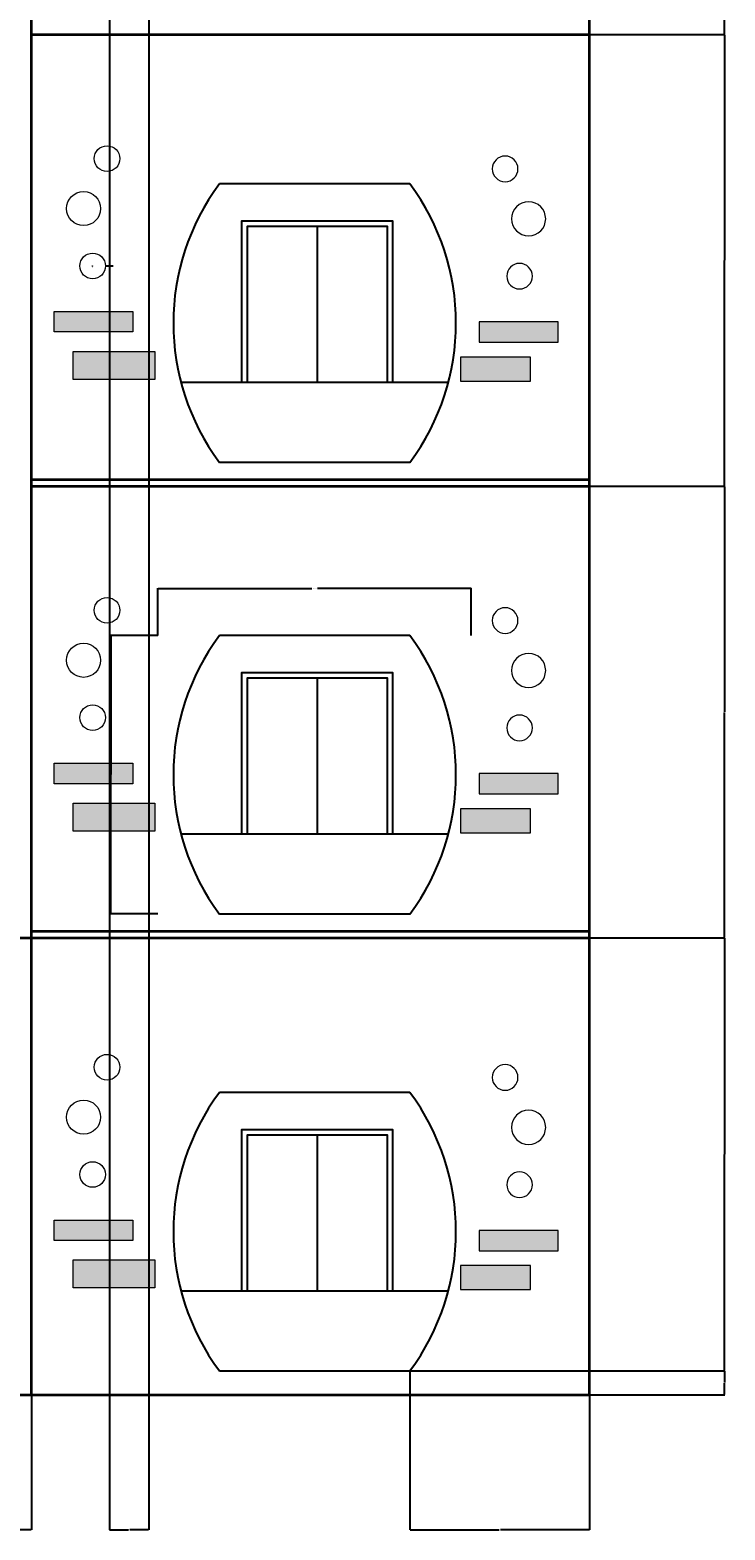
# Model space of a CAD drawing. Units: inches. Extents: x 328 to 2318, y 647 to 2548.
# Tile 3 of 5: x 1841 to 2318, y 696 to 1724. Entities that reach past the tile are written whole.
import ezdxf

# ---------------------------------------------------------------- set-up
doc = ezdxf.new("R2010")
doc.units = ezdxf.units.IN
doc.header["$MEASUREMENT"] = 0
for name, color, linetype, lineweight in [('A-ANNO-DIMS', 2, 'Continuous', 18), ('A-ELEV', 7, 'Continuous', 35), ('A-ELEV-ORNM', 7, 'Continuous', 18), ('A-GLAZ', 4, 'Continuous', 25)]:
    doc.layers.add(name, color=color, linetype=linetype, lineweight=lineweight)
doc.layers.add('A-ELEV-ORNM-PATT', color=18, linetype='Continuous', lineweight=13, true_color=0x000000)
doc.styles.get("Standard").update_dxf_attribs({"font": 'arial.ttf'})
doc.dimstyles.get("Standard").update_dxf_attribs({"dimtxt": 0.18, "dimasz": 0.18, "dimexe": 0.18, "dimexo": 0.0625, "dimgap": 0.09, "dimtad": 0, "dimtih": 1, "dimtoh": 1, "dimdec": 4, "dimzin": 0, "dimdsep": 46, "dimtxsty": 'Standard', "dimcen": 0.09, "dimadec": 0, "dimazin": 0, "dimtfac": 1, "dimtdec": 4, "dimtofl": 0, "dimtmove": 0, "dimatfit": 3, "dimfxl": 1, "dimtolj": 1, "dimtzin": 0, "dimarcsym": 0})

# ---------------------------------------------------------------- blocks, each defined once
blk = doc.blocks.new('WIN-ELEV-CURVED-SURROUND')
for p, q in [((162.1, 190.7), (31.6, 190.7)), ((98.6, 161.4), (98.6, 54.8)), ((5.2, 54.8), (188.5, 54.8)), ((31.6, 0), (162.1, 0))]:
    blk.add_line(p, q)
for points in [[(150.5, 54.8), (150.5, 165.1), (46.8, 165.1), (46.8, 54.8)], [(146.8, 54.8), (146.8, 161.4), (50.5, 161.4), (50.5, 54.8)]]:
    blk.add_lwpolyline(points)
for centre, start, end in [((159.8, 95.3), 143.3588, 216.6412), ((33.9, 95.3), 323.3588, 36.6412)]:
    blk.add_arc(centre, 159.8, start, end)
blk = doc.blocks.new('FACADE-THREE-ROUNDELS')
for centre, radius in [((27.8, 82.3), 8.8), ((11.7, 48.1), 11.7), ((17.9, 8.8), 8.77)]:
    blk.add_circle(centre, radius)
blk = doc.blocks.new('*D5')
at = {"layer": 'A-ANNO-DIMS', "color": 0, "lineweight": -2, "transparency": 16777216}
for p, q in [((1929.1, 1308.9), (1929.1, 1341.2)), ((1929.3, 1341), (2034.6, 1341)), ((2143.7, 1341), (2038.4, 1341)), ((2143.9, 1308.9), (2143.9, 1341.2))]:
    blk.add_line(p, q, dxfattribs=at)
at = {"layer": 'A-ANNO-DIMS', "color": 0, "transparency": 16777216}
for points in [[(1929.3, 1341.1), (1929.3, 1341), (1929.1, 1341)], [(2143.7, 1341.1), (2143.7, 1341), (2143.9, 1341)]]:
    blk.add_solid(points, dxfattribs=at)
at = {"layer": 'Defpoints', "color": 0, "transparency": 16777216}
for p in [(2143.9, 1341), (1929.1, 1308.8), (2143.9, 1308.8)]:
    blk.add_point(p, dxfattribs=at)
at = {"layer": 'A-ANNO-DIMS', "color": 0, "transparency": 16777216, "insert": (2036.5, 1341), "char_height": 0.18, "attachment_point": 5}
blk.add_mtext('\\A1;CURVED SURROUND 215 TYP.', dxfattribs=at)
blk = doc.blocks.new('*D6')
at = {"layer": 'A-ANNO-DIMS', "color": 0, "lineweight": -2, "transparency": 16777216}
for p, q in [((1929.1, 1308.8), (1896.8, 1308.8)), ((1896.9, 1308.6), (1896.9, 1213.7)), ((1896.9, 1118.3), (1896.9, 1213.3)), ((1929.1, 1118.1), (1896.8, 1118.1))]:
    blk.add_line(p, q, dxfattribs=at)
at = {"layer": 'A-ANNO-DIMS', "color": 0, "transparency": 16777216}
for points in [[(1896.9, 1308.6), (1897, 1308.6), (1896.9, 1308.8)], [(1896.9, 1118.3), (1897, 1118.3), (1896.9, 1118.1)]]:
    blk.add_solid(points, dxfattribs=at)
at = {"layer": 'Defpoints', "color": 0, "transparency": 16777216}
for p in [(1896.9, 1308.8), (1929.1, 1308.8), (1929.1, 1118.1)]:
    blk.add_point(p, dxfattribs=at)
at = {"layer": 'A-ANNO-DIMS', "color": 0, "transparency": 16777216, "insert": (1896.9, 1213.5), "char_height": 0.18, "attachment_point": 5}
blk.add_mtext('\\A1;191 TYP.', dxfattribs=at)
blk = doc.blocks.new('*D43')
at = {"layer": 'A-ANNO-DIMS', "color": 0, "lineweight": -2, "transparency": 16777216}
for p, q in [((2225, 1101.7), (2317.6, 1101.7)), ((2317.4, 1101.5), (2317.4, 953.6)), ((2317.4, 805.4), (2317.4, 953.3)), ((2101.8, 805.2), (2317.6, 805.2))]:
    blk.add_line(p, q, dxfattribs=at)
at = {"layer": 'A-ANNO-DIMS', "color": 0, "transparency": 16777216}
for points in [[(2317.4, 1101.5), (2317.5, 1101.5), (2317.4, 1101.7)], [(2317.4, 805.4), (2317.5, 805.4), (2317.4, 805.2)]]:
    blk.add_solid(points, dxfattribs=at)
at = {"layer": 'Defpoints', "color": 0, "transparency": 16777216}
for p in [(2225, 1101.7), (2317.4, 1101.7), (2101.8, 805.2)]:
    blk.add_point(p, dxfattribs=at)
at = {"layer": 'A-ANNO-DIMS', "color": 0, "transparency": 16777216, "insert": (2317.4, 953.5), "char_height": 0.18, "attachment_point": 5}
blk.add_mtext('\\A1;296.5', dxfattribs=at)
blk = doc.blocks.new('*D44')
at = {"layer": 'A-ANNO-DIMS', "color": 0, "lineweight": -2, "transparency": 16777216}
for p, q in [((2225, 1411.1), (2317.6, 1411.1)), ((2317.4, 1410.9), (2317.4, 1256.6)), ((2317.4, 1101.9), (2317.4, 1256.2)), ((2225, 1101.7), (2317.6, 1101.7))]:
    blk.add_line(p, q, dxfattribs=at)
at = {"layer": 'A-ANNO-DIMS', "color": 0, "transparency": 16777216}
for points in [[(2317.4, 1410.9), (2317.5, 1410.9), (2317.4, 1411.1)], [(2317.4, 1101.9), (2317.5, 1101.9), (2317.4, 1101.7)]]:
    blk.add_solid(points, dxfattribs=at)
at = {"layer": 'Defpoints', "color": 0, "transparency": 16777216}
for p in [(2225, 1411.1), (2317.4, 1411.1), (2225, 1101.7)]:
    blk.add_point(p, dxfattribs=at)
at = {"layer": 'A-ANNO-DIMS', "color": 0, "transparency": 16777216, "insert": (2317.4, 1256.4), "char_height": 0.18, "attachment_point": 5}
blk.add_mtext('\\A1;309.4', dxfattribs=at)
blk = doc.blocks.new('*D45')
at = {"layer": 'A-ANNO-DIMS', "color": 0, "lineweight": -2, "transparency": 16777216}
for p, q in [((2225, 1720.5), (2317.6, 1720.5)), ((2317.4, 1720.3), (2317.4, 1566)), ((2317.4, 1411.3), (2317.4, 1565.6)), ((2225, 1411.1), (2317.6, 1411.1))]:
    blk.add_line(p, q, dxfattribs=at)
at = {"layer": 'A-ANNO-DIMS', "color": 0, "transparency": 16777216}
for points in [[(2317.4, 1720.3), (2317.5, 1720.3), (2317.4, 1720.5)], [(2317.4, 1411.3), (2317.5, 1411.3), (2317.4, 1411.1)]]:
    blk.add_solid(points, dxfattribs=at)
at = {"layer": 'Defpoints', "color": 0, "transparency": 16777216}
for p in [(2225, 1720.5), (2317.4, 1720.5), (2225, 1411.1)]:
    blk.add_point(p, dxfattribs=at)
at = {"layer": 'A-ANNO-DIMS', "color": 0, "transparency": 16777216, "insert": (2317.4, 1565.8), "char_height": 0.18, "attachment_point": 5}
blk.add_mtext('\\A1;309.4', dxfattribs=at)
blk = doc.blocks.new('*D46')
at = {"layer": 'A-ANNO-DIMS', "color": 0, "lineweight": -2, "transparency": 16777216}
for p, q in [((2225, 2029.8), (2317.6, 2029.8)), ((2317.4, 2029.7), (2317.4, 1875.3)), ((2317.4, 1720.6), (2317.4, 1875)), ((2225, 1720.5), (2317.6, 1720.5))]:
    blk.add_line(p, q, dxfattribs=at)
at = {"layer": 'A-ANNO-DIMS', "color": 0, "transparency": 16777216}
for points in [[(2317.4, 2029.7), (2317.5, 2029.7), (2317.4, 2029.8)], [(2317.4, 1720.6), (2317.5, 1720.6), (2317.4, 1720.5)]]:
    blk.add_solid(points, dxfattribs=at)
at = {"layer": 'Defpoints', "color": 0, "transparency": 16777216}
for p in [(2225, 2029.8), (2317.4, 2029.8), (2225, 1720.5)]:
    blk.add_point(p, dxfattribs=at)
at = {"layer": 'A-ANNO-DIMS', "color": 0, "transparency": 16777216, "insert": (2317.4, 1875.1), "char_height": 0.18, "attachment_point": 5}
blk.add_mtext('\\A1;309.4', dxfattribs=at)
blk = doc.blocks.new('*D54')
at = {"layer": 'A-ANNO-DIMS', "color": 0, "lineweight": -2, "transparency": 16777216}
for p, q in [((2101.8, 805.1), (2101.8, 696.2)), ((2225, 788.7), (2225, 696.2)), ((2102, 696.3), (2163, 696.3)), ((2224.8, 696.3), (2163.8, 696.3))]:
    blk.add_line(p, q, dxfattribs=at)
at = {"layer": 'A-ANNO-DIMS', "color": 0, "transparency": 16777216}
for points in [[(2102, 696.4), (2102, 696.3), (2101.8, 696.3)], [(2224.8, 696.4), (2224.8, 696.3), (2225, 696.3)]]:
    blk.add_solid(points, dxfattribs=at)
at = {"layer": 'Defpoints', "color": 0, "transparency": 16777216}
for p in [(2101.8, 805.2), (2225, 788.8), (2101.8, 696.3)]:
    blk.add_point(p, dxfattribs=at)
at = {"layer": 'A-ANNO-DIMS', "color": 0, "transparency": 16777216, "insert": (2163.4, 696.3), "char_height": 0.18, "attachment_point": 5}
blk.add_mtext('\\A1;123.2', dxfattribs=at)
blk = doc.blocks.new('*D55')
at = {"layer": 'A-ANNO-DIMS', "color": 0, "lineweight": -2, "transparency": 16777216}
for p, q in [((2101.8, 805.2), (2317.6, 805.2)), ((2317.4, 805), (2317.4, 797.2)), ((2317.4, 789), (2317.4, 796.8)), ((2225, 788.8), (2317.6, 788.8))]:
    blk.add_line(p, q, dxfattribs=at)
at = {"layer": 'A-ANNO-DIMS', "color": 0, "transparency": 16777216}
for points in [[(2317.4, 805), (2317.5, 805), (2317.4, 805.2)], [(2317.4, 789), (2317.5, 789), (2317.4, 788.8)]]:
    blk.add_solid(points, dxfattribs=at)
at = {"layer": 'Defpoints', "color": 0, "transparency": 16777216}
for p in [(2101.8, 805.2), (2317.4, 805.2), (2225, 788.8)]:
    blk.add_point(p, dxfattribs=at)
at = {"layer": 'A-ANNO-DIMS', "color": 0, "transparency": 16777216, "insert": (2317.4, 797), "char_height": 0.18, "attachment_point": 5}
blk.add_mtext('\\A1;16.415', dxfattribs=at)
blk = doc.blocks.new('*D57')
at = {"layer": 'A-ANNO-DIMS', "color": 0, "lineweight": -2, "transparency": 16777216}
for p, q in [((1620, 788.7), (1620, 696.2)), ((1842.4, 788.7), (1842.4, 696.2)), ((1620.2, 696.3), (1730.9, 696.3)), ((1842.3, 696.3), (1731.6, 696.3))]:
    blk.add_line(p, q, dxfattribs=at)
at = {"layer": 'A-ANNO-DIMS', "color": 0, "transparency": 16777216}
for points in [[(1620.2, 696.4), (1620.2, 696.3), (1620, 696.3)], [(1842.3, 696.4), (1842.3, 696.3), (1842.4, 696.3)]]:
    blk.add_solid(points, dxfattribs=at)
at = {"layer": 'Defpoints', "color": 0, "transparency": 16777216}
for p in [(1620, 788.8), (1842.4, 788.8), (1620, 696.3)]:
    blk.add_point(p, dxfattribs=at)
at = {"layer": 'A-ANNO-DIMS', "color": 0, "transparency": 16777216, "insert": (1731.2, 696.3), "char_height": 0.18, "attachment_point": 5}
blk.add_mtext('\\A1;222.4', dxfattribs=at)
blk = doc.blocks.new('*D61')
at = {"layer": 'A-ANNO-DIMS', "color": 0, "lineweight": -2, "transparency": 16777216}
for p, q in [((1895.8, 2322.7), (1895.8, 696.2)), ((1922.9, 2242.4), (1922.9, 696.2)), ((1895.9, 696.3), (1908.9, 696.3)), ((1922.7, 696.3), (1909.8, 696.3))]:
    blk.add_line(p, q, dxfattribs=at)
at = {"layer": 'A-ANNO-DIMS', "color": 0, "transparency": 16777216}
for points in [[(1895.9, 696.4), (1895.9, 696.3), (1895.8, 696.3)], [(1922.7, 696.4), (1922.7, 696.3), (1922.9, 696.3)]]:
    blk.add_solid(points, dxfattribs=at)
at = {"layer": 'Defpoints', "color": 0, "transparency": 16777216}
for p in [(1895.8, 2322.7), (1922.9, 2242.4), (1895.8, 696.3)]:
    blk.add_point(p, dxfattribs=at)
at = {"layer": 'A-ANNO-DIMS', "color": 0, "transparency": 16777216, "insert": (1909.3, 696.3), "char_height": 0.18, "attachment_point": 5}
blk.add_mtext('\\A1;27.154', dxfattribs=at)
blk = doc.blocks.new('*D71')
at = {"layer": 'A-ANNO-DIMS', "color": 0, "lineweight": -2, "transparency": 16777216}
for p, q in [((1884.2, 1561.9), (1884.4, 1561.9)), ((1884.3, 1561.8), (1884.3, 1562)), ((1898.3, 1561.9), (1893.3, 1561.9))]:
    blk.add_line(p, q, dxfattribs=at)
at = {"layer": 'A-ANNO-DIMS', "color": 0, "transparency": 16777216}
blk.add_solid([(1893.3, 1561.9), (1893.3, 1561.9), (1893.1, 1561.9)], dxfattribs=at)
at = {"layer": 'Defpoints', "color": 0, "transparency": 16777216}
for p in [(1875.5, 1561.9), (1893.1, 1561.9)]:
    blk.add_point(p, dxfattribs=at)
at = {"layer": 'A-ANNO-DIMS', "color": 0, "transparency": 16777216, "insert": (1899.1, 1561.9), "char_height": 0.18, "attachment_point": 5}
blk.add_mtext('\\A1;16X ∅17.546', dxfattribs=at)

msp = doc.modelspace()

# ---------------------------------------------------------------- hatches: boundary and pattern name
at = {"layer": 'A-ELEV-ORNM-PATT'}
h = msp.add_hatch(color=256, dxfattribs=at)
h.dxf.hatch_style = 1
h.paths.add_polyline_path([(1160.8736, 1194.017), (1104.946, 1194.017), (1104.946, 1174.8467), (1160.8736, 1174.8467)])
h.paths.add_polyline_path([(1145.9162, 1221.3103), (1091.9395, 1221.3103), (1091.9395, 1207.3388), (1145.9162, 1207.3388)])
h.paths.add_polyline_path([(1418.337, 1190.1501), (1370.4156, 1190.1501), (1370.4156, 1173.7241), (1418.337, 1173.7241)])
h.paths.add_polyline_path([(1437.3105, 1214.299), (1383.3339, 1214.299), (1383.3339, 1200.3274), (1437.3105, 1200.3274)])
h.paths.add_polyline_path([(1418.337, 1499.5227), (1370.4156, 1499.5227), (1370.4156, 1483.0967), (1418.337, 1483.0967)])
h.paths.add_polyline_path([(1437.3105, 1523.6716), (1383.3339, 1523.6716), (1383.3339, 1509.7), (1437.3105, 1509.7)])
h.paths.add_polyline_path([(1145.9162, 1530.683), (1091.9395, 1530.683), (1091.9395, 1516.7114), (1145.9162, 1516.7114)])
h.paths.add_polyline_path([(1160.8736, 1503.3896), (1104.946, 1503.3896), (1104.946, 1484.2194), (1160.8736, 1484.2194)])
h.paths.add_polyline_path([(1160.8736, 1812.7623), (1104.946, 1812.7623), (1104.946, 1793.592), (1160.8736, 1793.592)])
h.paths.add_polyline_path([(1145.9162, 1840.0556), (1091.9395, 1840.0556), (1091.9395, 1826.084), (1145.9162, 1826.084)])
h.paths.add_polyline_path([(1437.3105, 1833.0442), (1383.3339, 1833.0442), (1383.3339, 1819.0726), (1437.3105, 1819.0726)])
h.paths.add_polyline_path([(1418.337, 1808.8953), (1370.4156, 1808.8953), (1370.4156, 1792.4693), (1418.337, 1792.4693)])
h.paths.add_polyline_path([(1145.9162, 908.3867), (1091.9395, 908.3867), (1091.9395, 894.4151), (1145.9162, 894.4151)])
h.paths.add_polyline_path([(1160.8736, 881.0933), (1104.946, 881.0933), (1104.946, 861.923), (1160.8736, 861.923)])
h.paths.add_polyline_path([(1418.337, 877.2264), (1370.4156, 877.2264), (1370.4156, 860.8004), (1418.337, 860.8004)])
h.paths.add_polyline_path([(1437.3105, 901.3753), (1383.3339, 901.3753), (1383.3339, 887.4037), (1437.3105, 887.4037)])
h.paths.add_polyline_path([(1926.897, 881.0933), (1870.9694, 881.0933), (1870.9694, 861.923), (1926.897, 861.923)])
h.paths.add_polyline_path([(1911.9396, 908.3867), (1857.9629, 908.3867), (1857.9629, 894.4151), (1911.9396, 894.4151)])
h.paths.add_polyline_path([(2184.3603, 877.2264), (2136.439, 877.2264), (2136.439, 860.8004), (2184.3603, 860.8004)])
h.paths.add_polyline_path([(2203.3339, 901.3753), (2149.3572, 901.3753), (2149.3572, 887.4037), (2203.3339, 887.4037)])
h.paths.add_polyline_path([(2184.3603, 1190.1501), (2136.439, 1190.1501), (2136.439, 1173.7241), (2184.3603, 1173.7241)])
h.paths.add_polyline_path([(2203.3339, 1214.299), (2149.3572, 1214.299), (2149.3572, 1200.3274), (2203.3339, 1200.3274)])
h.paths.add_polyline_path([(1911.9396, 1221.3103), (1857.9629, 1221.3103), (1857.9629, 1207.3388), (1911.9396, 1207.3388)])
h.paths.add_polyline_path([(1926.897, 1194.017), (1870.9694, 1194.017), (1870.9694, 1174.8467), (1926.897, 1174.8467)])
h.paths.add_polyline_path([(1926.897, 1503.3896), (1870.9694, 1503.3896), (1870.9694, 1484.2194), (1926.897, 1484.2194)])
h.paths.add_polyline_path([(1911.9396, 1530.683), (1857.9629, 1530.683), (1857.9629, 1516.7114), (1911.9396, 1516.7114)])
h.paths.add_polyline_path([(2184.3603, 1499.5227), (2136.439, 1499.5227), (2136.439, 1483.0967), (2184.3603, 1483.0967)])
h.paths.add_polyline_path([(2203.3339, 1523.6716), (2149.3572, 1523.6716), (2149.3572, 1509.7), (2203.3339, 1509.7)])
h.paths.add_polyline_path([(1926.897, 1812.7623), (1870.9694, 1812.7623), (1870.9694, 1793.592), (1926.897, 1793.592)])
h.paths.add_polyline_path([(1911.9396, 1840.0556), (1857.9629, 1840.0556), (1857.9629, 1826.084), (1911.9396, 1826.084)])
h.paths.add_polyline_path([(2184.3603, 1808.8953), (2136.439, 1808.8953), (2136.439, 1792.4693), (2184.3603, 1792.4693)])
h.paths.add_polyline_path([(2203.3339, 1833.0442), (2149.3572, 1833.0442), (2149.3572, 1819.0726), (2203.3339, 1819.0726)])

# ---------------------------------------------------------------- linework, layer by layer
at = {"layer": 'A-ELEV'}
for p, q in [((1842.45, 788.791), (1842.45, 2242.4288)), ((2224.9815, 788.791), (2224.9815, 2069.5914)), ((1842.45, 1720.4599), (2224.9815, 1720.4599)), ((1842.45, 1415.667), (2224.9815, 1415.667)), ((1842.45, 1411.0873), (2224.9815, 1411.0873)), ((1076.4266, 1101.7147), (2224.9815, 1101.7147)), ((1842.45, 1106.2944), (2224.9815, 1106.2944)), ((1121.2827, 788.791), (2224.9815, 788.791))]:
    msp.add_line(p, q, dxfattribs=at)
at = {"layer": 'A-ELEV-ORNM'}
for points in [[(1857.9629, 1530.683), (1911.9396, 1530.683), (1911.9396, 1516.7114), (1857.9629, 1516.7114)], [(2203.3339, 1523.6716), (2149.3572, 1523.6716), (2149.3572, 1509.7), (2203.3339, 1509.7)], [(1870.9694, 1503.3896), (1926.897, 1503.3896), (1926.897, 1484.2194), (1870.9694, 1484.2194)], [(2184.3603, 1499.5227), (2136.439, 1499.5227), (2136.439, 1483.0967), (2184.3603, 1483.0967)], [(1857.9629, 1221.3103), (1911.9396, 1221.3103), (1911.9396, 1207.3388), (1857.9629, 1207.3388)], [(2203.3339, 1214.299), (2149.3572, 1214.299), (2149.3572, 1200.3274), (2203.3339, 1200.3274)], [(1870.9694, 1194.017), (1926.897, 1194.017), (1926.897, 1174.8467), (1870.9694, 1174.8467)], [(2184.3603, 1190.1501), (2136.439, 1190.1501), (2136.439, 1173.7241), (2184.3603, 1173.7241)], [(1857.9629, 908.3867), (1911.9396, 908.3867), (1911.9396, 894.4151), (1857.9629, 894.4151)], [(2203.3339, 901.3753), (2149.3572, 901.3753), (2149.3572, 887.4037), (2203.3339, 887.4037)], [(1870.9694, 881.0933), (1926.897, 881.0933), (1926.897, 861.923), (1870.9694, 861.923)], [(2184.3603, 877.2264), (2136.439, 877.2264), (2136.439, 860.8004), (2184.3603, 860.8004)]]:
    msp.add_lwpolyline(points, close=True, dxfattribs=at)

# ---------------------------------------------------------------- block references
for p in [(1866.4251, 1553.1455), (1866.4251, 1243.7728), (1866.4251, 930.8492)]:
    msp.add_blockref('FACADE-THREE-ROUNDELS', p, dxfattribs=at)
at = {"layer": 'A-ELEV-ORNM', "extrusion": (0, 0, -1), "zscale": -1}
for p in [(-2194.8717, 1546.1341), (-2194.8717, 1236.7615), (-2194.8717, 923.8378)]:
    msp.add_blockref('FACADE-THREE-ROUNDELS', p, dxfattribs=at)
at = {"layer": 'A-GLAZ'}
for p in [(1939.6727, 1427.5026), (1939.6727, 1118.13), (1939.6727, 805.2063)]:
    msp.add_blockref('WIN-ELEV-CURVED-SURROUND', p, dxfattribs=at)

# ---------------------------------------------------------------- dimensions: what is measured, and where the dimension line sits
at = {"layer": 'A-ANNO-DIMS'}
for base, p1, p2, override, picture, middle in [((1895.76968, 696.34097), (1922.92323, 2242.42884), (1895.76968, 2322.73649), {"dimdec": 3, "dimlfac": 1, "dimrnd": 0, "dimzin": 0, "dimdsep": 46, "dimlunit": 2}, '*D61', (1909.34646, 696.34097)), ((2101.7855, 696.341), (2224.9815, 788.791), (2101.7855, 805.2063), {"dimdec": 1, "dimlfac": 1, "dimrnd": 0, "dimzin": 0, "dimdsep": 46, "dimlunit": 2}, '*D54', (2163.3835, 696.341))]:
    dim = msp.add_linear_dim(base=base, p1=p1, p2=p2, dimstyle='Standard', override=override, dxfattribs=at)
    dim.commit()
    dim.dimension.update_dxf_attribs({"geometry": picture, "text_midpoint": middle})
for base, p1, p2, angle, override, picture, middle in [((2317.4315, 2029.8325), (2224.9815, 1720.4599), (2224.9815, 2029.8325), 90, {"dimdec": 1, "dimlfac": 1, "dimrnd": 0, "dimzin": 0, "dimdsep": 46, "dimlunit": 2}, '*D46', (2317.4315, 1875.1462)), ((2317.4315, 1720.4599), (2224.9815, 1411.0873), (2224.9815, 1720.4599), 90, {"dimdec": 1, "dimlfac": 1, "dimrnd": 0, "dimzin": 0, "dimdsep": 46, "dimlunit": 2}, '*D45', (2317.4315, 1565.7736)), ((2317.4315, 1411.0873), (2224.9815, 1101.7147), (2224.9815, 1411.0873), 90, {"dimdec": 1, "dimlfac": 1, "dimrnd": 0, "dimzin": 0, "dimdsep": 46, "dimlunit": 2}, '*D44', (2317.4315, 1256.401)), ((2317.4315, 1101.7147), (2101.7855, 805.2063), (2224.9815, 1101.7147), 90, {"dimdec": 1, "dimlfac": 1, "dimrnd": 0, "dimzin": 0, "dimdsep": 46, "dimlunit": 2}, '*D43', (2317.4315, 953.4605)), ((2317.4315, 805.2063), (2224.9815, 788.791), (2101.7855, 805.2063), 90, {"dimdec": 3, "dimlfac": 1, "dimrnd": 0, "dimzin": 0, "dimdsep": 46, "dimlunit": 2}, '*D55', (2317.4315, 796.9987)), ((1620.0467, 696.341), (1842.45, 788.791), (1620.0467, 788.791), 180, {"dimdec": 1, "dimlfac": 1, "dimrnd": 0, "dimzin": 0, "dimdsep": 46, "dimlunit": 2}, '*D57', (1731.2483, 696.341))]:
    dim = msp.add_linear_dim(base=base, p1=p1, p2=p2, angle=angle, dimstyle='Standard', override=override, dxfattribs=at)
    dim.commit()
    dim.dimension.update_dxf_attribs({"geometry": picture, "text_midpoint": middle})
dim = msp.add_diameter_dim_2p(p1=(1875.5274, 1561.9187), p2=(1893.0731, 1561.918), text='16X <>', dimstyle='Standard', override={"dimdec": 3, "dimlfac": 1, "dimrnd": 0, "dimzin": 0, "dimdsep": 46, "dimlunit": 2}, dxfattribs=at)
dim.commit()
dim.dimension.update_dxf_attribs({"geometry": '*D71', "text_midpoint": (1898.3368, 1561.9178), "dimtype": 163})
dim = msp.add_linear_dim(base=(2143.8795, 1341.0301), p1=(1929.1492, 1308.8206), p2=(2143.8795, 1308.8206), text='CURVED SURROUND <> TYP.', dimstyle='Standard', override={"dimdec": 0, "dimlfac": 1, "dimrnd": 0, "dimzin": 0, "dimdsep": 46, "dimlunit": 2}, dxfattribs=at)
dim.commit()
dim.dimension.update_dxf_attribs({"geometry": '*D5', "text_midpoint": (2036.5144, 1341.0301)})
dim = msp.add_linear_dim(base=(1896.9397, 1308.8206), p1=(1929.1492, 1118.13), p2=(1929.1492, 1308.8206), angle=90, text='<> TYP.', dimstyle='Standard', override={"dimdec": 0, "dimlfac": 1, "dimrnd": 0, "dimzin": 0, "dimdsep": 46, "dimlunit": 2}, dxfattribs=at)
dim.commit()
dim.dimension.update_dxf_attribs({"geometry": '*D6', "text_midpoint": (1896.9397, 1213.4753)})

doc.saveas('drawing.dxf')
